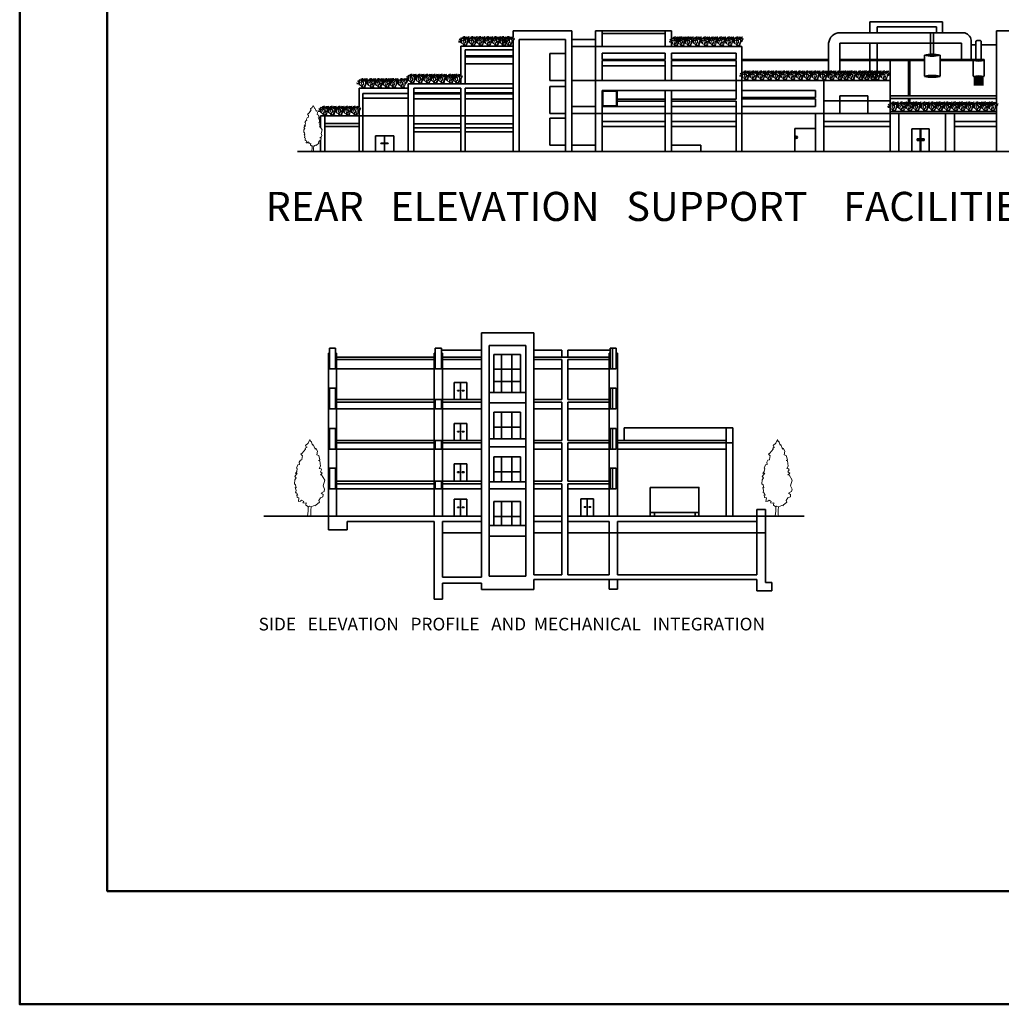
# Model space of a CAD drawing. Units: inches. Extents: x -1080 to 1950, y -1929 to 857.
# Tile 1 of 16: x -1080 to 294, y -1929 to -550. Entities that reach past the tile are written whole.
import ezdxf

# ---------------------------------------------------------------- set-up
doc = ezdxf.new("R2010")
doc.units = ezdxf.units.IN
doc.header["$MEASUREMENT"] = 0
for name, color, linetype, lineweight in [('A-ANNO-TEXT', 7, 'Continuous', 25), ('A-ANNO-TTLB', 7, 'Continuous', 50), ('A-ELEV', 7, 'Continuous', 35), ('L-PLNT', 82, 'Continuous', 13)]:
    doc.layers.add(name, color=color, linetype=linetype, lineweight=lineweight)
doc.styles.get("Standard").update_dxf_attribs({"font": 'arial.ttf'})

# ---------------------------------------------------------------- blocks, each defined once
blk = doc.blocks.new('*U6')
for p, q in [((-290.3982, 464.5406), (-265.6078, 577.8246)), ((-451.104, 219.456), (-601.0402, 303.8094)), ((-451.104, 219.456), (-587.4512, 234.2388)), ((-463.296, 280.416), (-552.577, 423.037)), ((-463.296, 280.416), (-512.064, 292.608)), ((-329.184, 316.992), (-499.872, 414.528)), ((-353.568, 316.992), (-487.68, 377.952)), ((-426.72, 414.528), (-475.488, 475.488)), ((-402.336, 207.264), (-463.296, 280.416)), ((-414.528, 182.88), (-463.296, 182.88)), ((-377.952, 463.296), (-451.104, 487.68)), ((-426.72, 316.992), (-451.104, 329.184)), ((-377.952, 146.304), (-451.104, 219.456)), ((-402.336, 12.192), (-451.104, 0)), ((-426.72, 414.528), (-390.144, 499.872)), ((-426.72, 316.992), (-426.72, 414.528)), ((-402.336, 207.264), (-426.72, 316.992)), ((-377.952, 146.304), (-402.336, 207.264)), ((-341.376, 12.192), (-402.336, 12.192)), ((-377.952, 463.296), (-329.184, 524.256)), ((-207.264, 304.8), (-377.952, 463.296)), ((-329.184, 121.92), (-377.952, 146.304)), ((-329.184, 316.992), (-353.568, 316.992)), ((-243.84, 24.384), (-341.376, 12.192)), ((-338.455, 424.7896), (-290.3982, 464.5406)), ((-329.184, 316.992), (-207.264, 451.104)), ((-268.224, 109.728), (-329.184, 316.992)), ((-292.608, 60.96), (-329.184, 121.92)), ((-243.84, 24.384), (-329.184, 0)), ((-316.7634, 502.285), (-327.6092, 559.9176)), ((-296.5958, 484.4034), (-316.7634, 502.285)), ((-286.512, 498.3226), (-307.4416, 538.0736)), ((-305.8922, 396.9512), (-302.7934, 478.4344)), ((-304.3428, 426.7708), (-268.7066, 458.5716)), ((-302.7934, 478.4344), (-270.256, 518.1854)), ((-219.456, 24.384), (-292.608, 60.96)), ((-268.7066, 458.5716), (-250.0884, 500.3038)), ((-207.264, 451.104), (-268.224, 548.64)), ((-268.224, 109.728), (-219.456, 195.072)), ((-219.456, 48.768), (-268.224, 109.728)), ((-243.84, 24.384), (-195.072, 24.384)), ((-240.792, 502.285), (-228.3968, 573.8368)), ((-182.88, 499.872), (-219.456, 512.064)), ((-219.456, 195.072), (-207.264, 304.8)), ((-219.456, 24.384), (-109.728, 73.152)), ((-219.456, 24.384), (-158.496, 73.152)), ((-219.456, 24.384), (-219.456, 48.768)), ((-219.456, 24.384), (-73.152, 24.384)), ((-207.264, 451.104), (-134.112, 487.68)), ((-195.072, 316.992), (-182.88, 377.952)), ((-170.688, 219.456), (-195.072, 316.992)), ((-195.072, 24.384), (-158.496, 12.192)), ((-182.88, 499.872), (-158.496, 536.448)), ((-121.92, 414.528), (-182.88, 499.872)), ((-182.88, 377.952), (-97.536, 426.72)), ((-146.304, 134.112), (-170.688, 219.456)), ((-158.496, 73.152), (-146.304, 134.112)), ((-158.496, 12.192), (-85.344, 0)), ((-129.1844, 450.6214), (-140.0302, 542.036)), ((-134.112, 487.68), (-97.536, 548.64)), ((-85.7758, 389.001), (-129.1844, 452.6026)), ((-73.152, 329.184), (-109.728, 499.872)), ((-109.728, 73.152), (-48.768, 243.84)), ((-97.536, 426.72), (-24.384, 524.256)), ((-85.7758, 472.4908), (-73.3552, 548.005)), ((-70.2564, 426.7708), (-85.7758, 472.4908)), ((-85.344, 134.112), (-73.152, 329.184)), ((-73.152, 402.336), (-60.96, 512.064)), ((-24.384, 268.224), (-73.152, 402.336)), ((-73.152, 24.384), (0, 0)), ((-48.768, 243.84), (24.384, 304.8)), ((-12.9032, 555.9552), (-2.0574, 522.1732)), ((-12.192, 274.32), (8.7884, 335.3562)), ((-5.1562, 486.3846), (2.5908, 542.036)), ((8.7884, 335.3562), (-5.1562, 486.3846)), ((-3.6068, 492.3536), (14.986, 518.1854)), ((-0.508, 508.254), (22.7584, 536.067)), ((1.0414, 526.1356), (35.1536, 559.9176)), ((2.5908, 542.036), (21.209, 555.9552)), ((8.7884, 335.3562), (33.6042, 412.8516)), ((24.384, 304.8), (36.576, 390.144)), ((24.384, 304.8), (73.152, 377.952)), ((33.6042, 412.8516), (92.5068, 464.5406)), ((36.576, 390.144), (73.152, 438.912)), ((48.768, 341.376), (60.96, 390.144)), ((60.96, 390.144), (85.344, 414.528))]:
    blk.add_line(p, q)
blk = doc.blocks.new('*U5')
blk.add_lwpolyline([(-2.754, 191.699), (-6.78, 182.851), (-13.682, 176.953), (-11.956, 173.266), (-9.656, 172.529), (-14.257, 170.317), (-13.682, 167.368), (-21.733, 157.783), (-25.184, 154.834), (-21.158, 150.41), (-21.733, 147.461), (-22.884, 140.825), (-26.334, 140.087), (-29.21, 134.926), (-28.635, 129.028), (-32.661, 128.291), (-36.111, 120.18), (-34.386, 118.706), (-35.536, 111.333), (-38.987, 106.171), (-34.386, 107.646), (-40.712, 98.798), (-37.261, 95.849), (-40.712, 90.688), (-41.287, 80.366), (-38.412, 78.154), (-36.686, 70.781), (-39.562, 71.518), (-37.261, 64.145), (-38.412, 57.509), (-36.111, 58.247), (-33.236, 52.348), (-35.536, 53.086), (-34.961, 46.45), (-30.36, 44.975), (-31.51, 36.128), (-26.334, 36.865), (-23.459, 39.814), (-18.283, 36.128), (-20.008, 33.178), (-14.832, 31.704), (-11.956, 33.178), (-12.531, 27.28), (-6.205, 22.856), (-3.905, 24.331), (0.121, 22.856), (8.173, 26.543), (11.624, 25.068), (12.199, 27.28), (21.4, 34.653), (19.675, 39.077), (23.701, 44.975), (30.027, 47.924), (30.602, 53.823), (25.426, 56.772), (32.903, 61.196), (34.053, 67.094), (30.602, 75.205), (34.628, 89.951), (26.576, 103.222), (23.701, 103.222), (28.302, 107.646), (23.701, 110.595), (26.576, 115.756), (25.426, 117.968), (20.825, 118.706), (24.276, 124.604), (22.551, 137.876), (19.1, 139.35), (22.551, 140.825), (19.675, 151.884), (14.499, 153.359), (16.224, 162.207), (12.199, 170.317), (10.473, 167.368), (5.872, 179.165), (4.147, 177.69), (0.696, 187.275), (-0.454, 185.8)], close=True)
for points in [[(-6.813, 23.669), (-6.813, 11.669), (-8.627, 0)], [(0.387, 23.669), (-0.576, 13.271), (-0.576, 3.686), (0, 0)]]:
    blk.add_lwpolyline(points)

msp = doc.modelspace()

# ---------------------------------------------------------------- linework, layer by layer
at = {"layer": 'A-ANNO-TTLB'}
for points in [[(-1080.1, 856.5), (1950.4, 856.5), (1950.4, -1929), (-1080.1, -1929)], [(-957.6, 743.5), (1813.4, 743.5), (1813.4, -1770.5), (-957.6, -1770.5)]]:
    msp.add_lwpolyline(points, close=True, dxfattribs=at)
at = {"layer": 'A-ELEV'}
for p, q in [((-307.2, -565.3), (-389.4, -565.3)), ((-389.4, -565.3), (-389.4, -573.8)), ((-307.2, -734.7), (-307.2, -565.3)), ((-274.1, -565.3), (-264.9, -565.3)), ((-274.1, -565.3), (-274.1, -577.5)), ((-274.1, -565.3), (-176.6, -565.3)), ((-264.9, -587.2), (-264.9, -565.3)), ((-176.6, -565.3), (-176.6, -577.5)), ((-167.5, -565.3), (-176.6, -565.3)), ((-167.5, -576.3), (-167.5, -565.3)), ((109.9, -552.8), (211.8, -552.8)), ((109.9, -567.9), (109.9, -552.8)), ((120, -567.9), (120, -559.8)), ((120, -559.8), (203, -559.8)), ((203, -559.8), (203, -567.9)), ((211.8, -552.8), (211.8, -567.9)), ((287.1, -565.3), (287.1, -606)), ((287.1, -565.3), (345.7, -565.3)), ((-389.4, -574.1), (-389.4, -574.7)), ((-389.4, -578.7), (-389.4, -578.9)), ((-380.8, -734.7), (-380.8, -577.5)), ((-380.8, -577.5), (-315.9, -577.5)), ((-315.9, -577.5), (-315.9, -734.7)), ((-307.2, -577.5), (-274.1, -577.5)), ((-274.1, -577.5), (-274.1, -587.2)), ((-264.9, -569.2), (-176.6, -569.2)), ((-176.6, -577.5), (-176.6, -587.2)), ((68, -568.1), (114.5, -568.1)), ((109.9, -567.9), (109.9, -568.1)), ((114.5, -568.1), (240.5, -568.1)), ((120, -567.9), (120, -567.9)), ((120, -567.9), (120, -568.1)), ((194.9, -568.1), (194.9, -599.6)), ((198.9, -568.1), (198.9, -599.6)), ((203, -567.9), (203, -568.1)), ((211.8, -567.9), (211.8, -568.1)), ((251.9, -578.8), (251.9, -605.7)), ((-462.5, -587), (-389.4, -587)), ((-462.5, -628.8), (-462.5, -587)), ((-389.4, -592), (-456.5, -592)), ((-456.5, -639.5), (-456.5, -592)), ((-456.5, -592), (-389.4, -592)), ((-455.2, -592), (-389.4, -592)), ((-389.4, -579.9), (-389.4, -587)), ((-389.4, -587), (-389.4, -592)), ((-389.4, -592), (-389.4, -734.7)), ((-307.2, -587.2), (-274.1, -587.2)), ((-274.1, -587.2), (-274.1, -734.7)), ((-274.1, -587.2), (-167.5, -587.2)), ((-167.5, -581.8), (-167.5, -587.2)), ((-167.5, -587.2), (-77.3, -587.2)), ((-69.5, -587.2), (-77.3, -587.2)), ((-69.5, -623.6), (-69.5, -587.2)), ((52.2, -623.6), (52.2, -582.7)), ((68.1, -582.7), (114.5, -582.7)), ((68.1, -623.9), (68.1, -582.7)), ((109.9, -582.7), (109.9, -623.7)), ((109.9, -582.7), (109.9, -585.8)), ((114.5, -582.7), (238.3, -582.7)), ((120, -582.7), (120, -623.5)), ((120, -582.7), (120, -585.8)), ((238.3, -582.7), (238.3, -605.7)), ((251.9, -585), (258.5, -585)), ((258.5, -588.2), (258.5, -579.9)), ((258.5, -605.7), (258.5, -588.2)), ((265.9, -579.9), (265.9, -588.2)), ((265.9, -585), (287.1, -585)), ((265.9, -588.2), (265.9, -605.7)), ((-456.5, -600.7), (-389.4, -600.7)), ((-456.5, -601.9), (-389.4, -601.9)), ((-315.9, -597.3), (-338.1, -597.3)), ((-338.1, -597.3), (-338.1, -635.1)), ((-264.9, -596.9), (-176.6, -596.9)), ((-264.9, -605.7), (-264.9, -596.9)), ((-264.9, -605.7), (-176.6, -605.7)), ((-176.6, -596.9), (-176.6, -605.7)), ((-167.5, -596.9), (-77.3, -596.9)), ((-167.5, -596.9), (-167.5, -605.7)), ((-167.5, -605.7), (-77.3, -605.7)), ((-77.3, -596.9), (-77.3, -605.7)), ((-69.5, -605.7), (52.2, -605.7)), ((68.1, -605.7), (166.1, -605.7)), ((138.3, -635.1), (138.3, -605.7)), ((166.1, -605.7), (166.1, -656.7)), ((166.1, -605.7), (186.3, -605.7)), ((194.9, -599.6), (186.3, -599.6)), ((186.3, -599.6), (186.3, -629.2)), ((194.9, -599.6), (208.3, -599.6)), ((208.3, -629.2), (208.3, -599.6)), ((208.3, -605.7), (264.9, -605.7)), ((254.5, -605.7), (254.5, -629.2)), ((269.9, -605.7), (264.9, -605.7)), ((269.9, -605.7), (269.9, -607.2)), ((287.1, -665.7), (287.1, -606)), ((-456.5, -611.5), (-389.4, -611.5)), ((-264.9, -635.1), (-264.9, -607.2)), ((-264.9, -607.2), (-176.6, -607.2)), ((-264.9, -614.5), (-176.6, -614.5)), ((-176.6, -607.2), (-176.6, -635.1)), ((-167.5, -607.2), (-77.3, -607.2)), ((-167.5, -607.2), (-167.5, -635.1)), ((-167.5, -614.5), (-77.3, -614.5)), ((-77.3, -607.2), (-77.3, -661.3)), ((-69.5, -607.2), (52.2, -607.2)), ((68.1, -607.2), (164.1, -607.2)), ((164.1, -607.2), (164.1, -656.7)), ((164.1, -607.2), (186.3, -607.2)), ((208.3, -607.2), (254.5, -607.2)), ((254.5, -607.2), (269.9, -607.2)), ((269.9, -629.2), (269.9, -607.2)), ((-462.5, -639.5), (-462.5, -632.1)), ((-69.5, -628.1), (-69.5, -627.8)), ((-69.5, -659), (-69.5, -629.3)), ((52.2, -630.9), (52.2, -626.5)), ((68.1, -629.3), (68.1, -628.1)), ((68.1, -635.1), (68.1, -633.8)), ((109.9, -626.5), (109.9, -631.3)), ((120, -624.3), (120, -630.1)), ((120, -634.3), (120, -635.1)), ((186.3, -629.2), (208.3, -629.2)), ((256.6, -628.9), (256.6, -642.2)), ((258.1, -628.9), (258.1, -642.2)), ((259.2, -628.9), (259.2, -642.2)), ((260.7, -628.9), (260.7, -642.2)), ((262, -628.9), (262, -642.2)), ((263.4, -628.9), (263.4, -642.2)), ((263.4, -628.9), (263.4, -642.2)), ((264.7, -628.9), (264.7, -642.2)), ((265.7, -628.9), (265.7, -642.2)), ((266.8, -628.9), (266.8, -642.2)), ((268, -628.9), (268, -642.2)), ((268, -628.9), (268, -642.2)), ((-604.9, -657.6), (-604.9, -645.6)), ((-604.9, -645.6), (-536.5, -645.6)), ((-536.5, -645.6), (-536.5, -639.5)), ((-536.5, -639.5), (-528.2, -639.5)), ((-536.5, -653.1), (-536.5, -645.6)), ((-528.2, -639.5), (-462.5, -639.5)), ((-528.2, -639.5), (-462.5, -639.5)), ((-528.2, -734.7), (-528.2, -645.6)), ((-528.2, -645.6), (-462.5, -645.6)), ((-528.2, -645.6), (-462.5, -645.6)), ((-462.5, -639.5), (-389.4, -639.5)), ((-462.5, -734.7), (-462.5, -645.6)), ((-456.5, -645.6), (-456.5, -734.7)), ((-456.5, -645.6), (-389.4, -645.6)), ((-338.1, -635.1), (-315.9, -635.1)), ((-315.9, -643.6), (-338.1, -643.6)), ((-338.1, -643.6), (-338.1, -681.3)), ((-307.2, -635.1), (-77.3, -635.1)), ((-77.3, -635.1), (113, -635.1)), ((45.4, -734.7), (45.4, -635.1)), ((52.2, -635.1), (52.2, -634.6)), ((109.9, -634.6), (109.9, -635.1)), ((113, -635.1), (138.3, -635.1)), ((138.3, -635.1), (138.3, -667.8)), ((-604.9, -657.6), (-604.9, -672.3)), ((-600, -734.7), (-600, -653.1)), ((-536.5, -653.1), (-600, -653.1)), ((-600, -659.7), (-536.5, -659.7)), ((-536.5, -653.1), (-536.5, -734.7)), ((-528.2, -652.3), (-462.5, -652.3)), ((-528.2, -653.7), (-462.5, -653.7)), ((-528.2, -660.9), (-462.5, -660.9)), ((-456.5, -652.3), (-389.4, -652.3)), ((-456.5, -653.7), (-389.4, -653.7)), ((-456.5, -660.9), (-389.4, -660.9)), ((-264.9, -734), (-264.9, -649.2)), ((-264.9, -649.2), (-77.3, -649.2)), ((-244, -671.6), (-244, -649.2)), ((-244, -661.3), (-176.6, -661.3)), ((-176.6, -649.2), (-176.6, -734.7)), ((-167.5, -649.2), (-167.5, -661.3)), ((-167.5, -661.3), (-77.3, -661.3)), ((-167.5, -661.3), (-167.5, -734.7)), ((-69.5, -649.2), (34, -649.2)), ((-69.5, -659), (34, -659)), ((-69.5, -660.9), (-69.5, -659)), ((-69.5, -734.7), (-69.5, -660.9)), ((-69.5, -660.9), (34, -660.9)), ((34, -649.2), (34, -659)), ((34, -660.9), (34, -671.6)), ((68, -681.3), (68, -656.4)), ((68, -656.4), (107, -656.4)), ((107, -656.4), (107, -681.3)), ((138.3, -656.7), (287.1, -656.7)), ((138.3, -660.1), (287.1, -660.1)), ((164.1, -660.1), (164.1, -666.5)), ((166.1, -660.1), (166.1, -666.2)), ((-307.2, -671.6), (-274.1, -671.6)), ((-264.9, -671.6), (-176.6, -671.6)), ((-176.6, -663.9), (-244, -663.9)), ((-167.5, -663.9), (-77.3, -663.9)), ((-167.5, -671.6), (-77.3, -671.6)), ((-77.3, -663.9), (-77.3, -734.7)), ((34, -671.6), (-69.5, -671.6)), ((45.4, -663.4), (138.3, -663.4)), ((138.3, -669.1), (138.3, -670.5)), ((138.3, -674), (138.3, -734.7)), ((164.1, -667.2), (164.1, -667.8)), ((287.1, -681.3), (287.1, -670.8)), ((-659, -684.4), (-653.2, -684.4)), ((-659, -700.7), (-659, -684.4)), ((-653.2, -684.4), (-653.2, -734.7)), ((-653.2, -684.4), (-604.9, -684.4)), ((-604.9, -677.4), (-604.9, -684.4)), ((-604.9, -684.4), (-604.9, -734.7)), ((-604.9, -684.4), (-600, -684.4)), ((-600, -684.5), (-528.2, -684.5)), ((-528.2, -684.5), (-462.5, -684.5)), ((-462.5, -684.5), (-456.5, -684.5)), ((-456.5, -684.5), (-389.4, -684.5)), ((-338.1, -681.3), (-315.9, -681.3)), ((-315.9, -687.9), (-338.1, -687.9)), ((-338.1, -687.9), (-338.1, -725.6)), ((-307.2, -681.3), (-264.9, -681.3)), ((-264.9, -681.3), (-77.3, -681.3)), ((-77.3, -681.3), (93.5, -681.3)), ((34, -681.3), (34, -734.7)), ((93.5, -681.3), (138.3, -681.3)), ((138.3, -678.4), (287.1, -678.4)), ((138.3, -681.3), (228.4, -681.3)), ((150.7, -681.3), (150.7, -734.7)), ((164.1, -676.9), (164.1, -678.4)), ((166.1, -677.5), (166.1, -678.4)), ((215.6, -681.3), (215.6, -734.7)), ((228.4, -681.3), (228.4, -734.7)), ((228.4, -681.3), (287.1, -681.3)), ((287.1, -681.3), (287.1, -734.7)), ((-653.2, -695.5), (-604.9, -695.5)), ((-653.2, -699.7), (-604.9, -699.7)), ((-528.2, -695.7), (-462.5, -695.7)), ((-528.2, -701.4), (-462.5, -701.4)), ((-456.5, -695.7), (-389.4, -695.7)), ((-456.5, -701.4), (-389.4, -701.4)), ((-264.7, -692.6), (-176.6, -692.6)), ((-264.7, -699.5), (-176.6, -699.5)), ((-167.5, -692.6), (-77.3, -692.6)), ((-167.5, -699.5), (-77.3, -699.5)), ((34, -702.4), (4.7, -702.4)), ((4.7, -702.4), (4.7, -734.7)), ((45.4, -692.6), (138.3, -692.6)), ((45.4, -699.5), (138.3, -699.5)), ((168.5, -734.7), (168.5, -702.6)), ((168.5, -702.6), (192.9, -702.6)), ((180.3, -702.6), (180.3, -734.7)), ((181.2, -702.6), (181.2, -734.7)), ((192.9, -702.6), (192.9, -734.7)), ((228.4, -692.6), (287.1, -692.6)), ((228.4, -699.5), (287.1, -699.5)), ((-659, -716), (-659, -714.9)), ((-582.1, -734.7), (-582.1, -712.4)), ((-582.1, -712.4), (-556.3, -712.4)), ((-569.3, -712.4), (-569.3, -734.7)), ((-556.3, -712.4), (-556.3, -734.7)), ((-528.2, -707), (-462.5, -707)), ((-456.5, -707), (-389.4, -707)), ((6.9, -714.5), (7.7, -714.5)), ((176, -716.8), (176, -719.3)), ((179.7, -716.8), (176, -716.8)), ((179.7, -719.3), (179.7, -716.8)), ((182.1, -716.8), (182.1, -719.3)), ((185.9, -716.8), (182.1, -716.8)), ((185.9, -719.3), (185.9, -716.8)), ((-659, -718.2), (-659, -734.7)), ((-659, -734.7), (-659, -718.7)), ((-574.4, -723.5), (-574.4, -722.7)), ((-574.4, -722.7), (-573.3, -722.7)), ((-570.8, -723.5), (-574.4, -723.5)), ((-573.3, -722.7), (-570.8, -722.7)), ((-570.8, -722.7), (-570.8, -723.5)), ((-568.1, -723.5), (-568.1, -722.7)), ((-568.1, -722.7), (-566.9, -722.7)), ((-564.4, -723.5), (-568.1, -723.5)), ((-566.9, -722.7), (-564.4, -722.7)), ((-564.4, -722.7), (-564.4, -723.5)), ((-338.1, -725.6), (-315.9, -725.6)), ((-307.2, -725.6), (-274.1, -725.6)), ((-167.5, -725.6), (-126.7, -725.6)), ((-126.7, -725.6), (-126.7, -734.7)), ((176, -719.3), (179.7, -719.3)), ((182.1, -719.3), (185.9, -719.3)), ((-691.1, -734.7), (-262.7, -734.7)), ((-262.7, -734.7), (342.8, -734.7)), ((-433.5, -1258.6), (-433.5, -988.5)), ((-433.5, -988.5), (-360.3, -988.5)), ((-360.3, -988.5), (-360.3, -1327.4)), ((-422.8, -1329.4), (-422.8, -1006.4)), ((-422.8, -1006.4), (-371.6, -1006.4)), ((-371.6, -1006.4), (-371.6, -1329.4)), ((-647.8, -1245.3), (-647.8, -1017.1)), ((-647.8, -1017.1), (-646.5, -1017.1)), ((-646.5, -1017.1), (-646.5, -1009.9)), ((-646.5, -1009.9), (-638, -1009.9)), ((-646.5, -1017.1), (-646.5, -1038.8)), ((-638, -1009.9), (-638, -1017.1)), ((-638, -1038.8), (-638, -1017.1)), ((-638, -1017.1), (-636.5, -1017.1)), ((-636.5, -1017.1), (-636.5, -1245.3)), ((-499.7, -1245.3), (-499.7, -1017.1)), ((-499.7, -1017.1), (-498.4, -1017.1)), ((-498.4, -1017.1), (-498.4, -1009.9)), ((-498.4, -1009.9), (-489.9, -1009.9)), ((-498.4, -1017.1), (-498.4, -1038.8)), ((-489.9, -1009.9), (-489.9, -1017.1)), ((-489.9, -1012.9), (-433.5, -1012.9)), ((-489.9, -1017.1), (-488.3, -1017.1)), ((-489.9, -1038.8), (-489.9, -1017.1)), ((-488.3, -1017.1), (-488.3, -1245.3)), ((-416.3, -1072), (-416.3, -1018.6)), ((-416.3, -1018.6), (-379.2, -1018.6)), ((-405.8, -1018.6), (-405.8, -1072)), ((-391.4, -1018.6), (-391.4, -1072)), ((-379.2, -1018.6), (-379.2, -1072.2)), ((-360.3, -1012.9), (-321.1, -1012.9)), ((-321.1, -1012.9), (-321.1, -1022.5)), ((-312.8, -1012.9), (-312.8, -1022.5)), ((-312.8, -1012.9), (-253.6, -1012.9)), ((-254.9, -1245.3), (-254.9, -1017.1)), ((-254.9, -1017.1), (-253.6, -1017.1)), ((-253.6, -1017.1), (-253.6, -1009.9)), ((-253.6, -1009.9), (-245.1, -1009.9)), ((-253.6, -1017.1), (-253.6, -1038.8)), ((-250.1, -1009.9), (-250.1, -1038.8)), ((-245.1, -1009.9), (-245.1, -1017.1)), ((-245.1, -1017.1), (-243.5, -1017.1)), ((-245.1, -1038.8), (-245.1, -1017.1)), ((-243.5, -1017.1), (-243.5, -1245.3)), ((-636.5, -1022.5), (-498.4, -1022.5)), ((-636.5, -1025.8), (-498.4, -1025.8)), ((-489.9, -1022.5), (-433.5, -1022.5)), ((-489.9, -1025.8), (-433.5, -1025.8)), ((-360.3, -1022.5), (-321.1, -1022.5)), ((-360.3, -1025.8), (-321.1, -1025.8)), ((-321.1, -1022.5), (-312.8, -1022.5)), ((-321.1, -1025.8), (-321.1, -1082)), ((-312.8, -1022.5), (-254.9, -1022.5)), ((-312.8, -1025.8), (-254.9, -1025.8)), ((-312.8, -1025.8), (-312.8, -1082)), ((-646.5, -1038.8), (-638, -1038.8)), ((-638, -1038.8), (-433.5, -1038.8)), ((-498.4, -1038.8), (-489.9, -1038.8)), ((-416.3, -1039.3), (-379.2, -1039.3)), ((-360.3, -1038.8), (-321.1, -1038.8)), ((-312.8, -1038.8), (-254.9, -1038.8)), ((-253.6, -1038.8), (-245.1, -1038.8)), ((-471.8, -1082), (-471.8, -1058)), ((-471.8, -1058), (-454.2, -1058)), ((-462.9, -1082), (-462.9, -1058)), ((-454.2, -1058), (-454.2, -1082)), ((-416.3, -1056.7), (-379.2, -1056.7)), ((-646.5, -1073.3), (-646.5, -1066.1)), ((-646.5, -1066.1), (-638, -1066.1)), ((-646.5, -1073.3), (-646.5, -1095)), ((-638, -1066.1), (-638, -1073.3)), ((-638, -1095), (-638, -1073.3)), ((-467.4, -1069.1), (-467.4, -1069.8)), ((-464.8, -1069.1), (-467.4, -1069.1)), ((-467.4, -1069.8), (-464.8, -1069.8)), ((-464.8, -1069.8), (-464.8, -1069.1)), ((-460.7, -1069.1), (-460.7, -1069.8)), ((-458.1, -1069.1), (-460.7, -1069.1)), ((-460.7, -1069.8), (-458.1, -1069.8)), ((-458.1, -1069.8), (-458.1, -1069.1)), ((-422.8, -1072), (-371.6, -1072)), ((-253.6, -1073.3), (-253.6, -1066.1)), ((-253.6, -1066.1), (-245.1, -1066.1)), ((-253.6, -1073.3), (-253.6, -1095)), ((-250.1, -1066.1), (-250.1, -1095)), ((-245.1, -1066.1), (-245.1, -1073.3)), ((-245.1, -1095), (-245.1, -1073.3)), ((-636.5, -1082), (-499.7, -1082)), ((-636.5, -1085.5), (-499.7, -1085.5)), ((-498.4, -1082), (-498.4, -1095)), ((-498.4, -1082), (-489.9, -1082)), ((-489.9, -1095), (-489.9, -1082)), ((-488.3, -1082), (-433.5, -1082)), ((-488.3, -1085.5), (-433.5, -1085.5)), ((-422.8, -1086.5), (-371.6, -1086.5)), ((-360.3, -1082), (-321.1, -1082)), ((-360.3, -1085.5), (-321.1, -1085.5)), ((-321.1, -1085.5), (-321.1, -1139.5)), ((-312.8, -1082), (-254.9, -1082)), ((-312.8, -1085.5), (-254.9, -1085.5)), ((-312.8, -1085.5), (-312.8, -1139.5)), ((-646.5, -1095), (-638, -1095)), ((-638, -1095), (-499.7, -1095)), ((-498.4, -1095), (-489.9, -1095)), ((-498.4, -1095), (-489.9, -1095)), ((-488.3, -1095), (-433.5, -1095)), ((-416.3, -1099.8), (-379.2, -1099.8)), ((-416.3, -1137.1), (-416.3, -1099.8)), ((-405.8, -1099.8), (-405.8, -1137.1)), ((-391.4, -1099.8), (-391.4, -1137.1)), ((-379.2, -1099.8), (-379.2, -1137.1)), ((-360.3, -1095), (-321.1, -1095)), ((-312.8, -1095), (-254.9, -1095)), ((-253.6, -1095), (-245.1, -1095)), ((-471.8, -1139.5), (-471.8, -1115.5)), ((-471.8, -1115.5), (-454.2, -1115.5)), ((-462.9, -1139.5), (-462.9, -1115.5)), ((-454.2, -1115.5), (-454.2, -1139.5)), ((-646.5, -1129.5), (-646.5, -1122.3)), ((-646.5, -1122.3), (-638, -1122.3)), ((-646.5, -1129.5), (-646.5, -1151.2)), ((-638, -1122.3), (-638, -1129.5)), ((-638, -1151.2), (-638, -1129.5)), ((-467.4, -1126.6), (-467.4, -1127.3)), ((-464.8, -1126.6), (-467.4, -1126.6)), ((-467.4, -1127.3), (-464.8, -1127.3)), ((-464.8, -1127.3), (-464.8, -1126.6)), ((-460.7, -1126.6), (-460.7, -1127.3)), ((-458.1, -1126.6), (-460.7, -1126.6)), ((-460.7, -1127.3), (-458.1, -1127.3)), ((-458.1, -1127.3), (-458.1, -1126.6)), ((-416.3, -1120.5), (-379.2, -1120.5)), ((-253.6, -1129.5), (-253.6, -1122.3)), ((-253.6, -1122.3), (-245.1, -1122.3)), ((-253.6, -1129.5), (-253.6, -1151.2)), ((-250.1, -1122.3), (-250.1, -1151.2)), ((-245.1, -1122.3), (-245.1, -1129.5)), ((-245.1, -1151.2), (-245.1, -1129.5)), ((-234.2, -1139.3), (-234.2, -1121.4)), ((-234.2, -1121.4), (-81.7, -1121.4)), ((-91.3, -1124.9), (-91.3, -1121.4)), ((-91.3, -1142.7), (-91.3, -1124.9)), ((-81.7, -1121.4), (-81.7, -1124.9)), ((-81.7, -1124.9), (-81.7, -1245.3)), ((-636.5, -1139.5), (-499.7, -1139.5)), ((-636.5, -1142.7), (-499.7, -1142.7)), ((-498.4, -1139.5), (-498.4, -1151.2)), ((-498.4, -1139.5), (-489.9, -1139.5)), ((-489.9, -1151.2), (-489.9, -1139.5)), ((-488.3, -1139.5), (-433.5, -1139.5)), ((-488.3, -1142.7), (-433.5, -1142.7)), ((-422.8, -1137.1), (-371.6, -1137.1)), ((-360.3, -1139.5), (-321.1, -1139.5)), ((-360.3, -1142.7), (-321.1, -1142.7)), ((-321.1, -1142.7), (-321.1, -1196.1)), ((-312.8, -1139.5), (-254.9, -1139.5)), ((-312.8, -1142.7), (-254.9, -1142.7)), ((-312.8, -1142.7), (-312.8, -1196.1)), ((-243.5, -1139.3), (-178.2, -1139.3)), ((-243.5, -1142.7), (-91.3, -1142.7)), ((-178.2, -1139.3), (-91.3, -1139.3)), ((-91.3, -1142.7), (-81.7, -1142.7)), ((-91.3, -1142.7), (-91.3, -1245.3)), ((-646.5, -1151.2), (-638, -1151.2)), ((-638, -1151.2), (-499.7, -1151.2)), ((-498.4, -1151.2), (-489.9, -1151.2)), ((-498.4, -1151.2), (-489.9, -1151.2)), ((-488.3, -1151.2), (-433.5, -1151.2)), ((-422.8, -1148.2), (-371.6, -1148.2)), ((-360.3, -1151.2), (-321.1, -1151.2)), ((-312.8, -1151.2), (-254.9, -1151.2)), ((-253.6, -1151.2), (-245.1, -1151.2)), ((-243.5, -1151.2), (-91.3, -1151.2)), ((-471.8, -1196.1), (-471.8, -1172.1)), ((-471.8, -1172.1), (-454.2, -1172.1)), ((-462.9, -1196.1), (-462.9, -1172.1)), ((-454.2, -1172.1), (-454.2, -1196.1)), ((-416.3, -1197.2), (-416.3, -1162.3)), ((-416.3, -1162.3), (-379.2, -1162.3)), ((-405.8, -1162.3), (-405.8, -1197.2)), ((-391.4, -1162.3), (-391.4, -1197.2)), ((-379.2, -1162.3), (-379.2, -1197.2)), ((-646.5, -1185), (-646.5, -1177.8)), ((-646.5, -1177.8), (-638, -1177.8)), ((-646.5, -1185), (-646.5, -1206.8)), ((-638, -1177.8), (-638, -1185)), ((-638, -1206.8), (-638, -1185)), ((-467.4, -1183.2), (-467.4, -1183.9)), ((-464.8, -1183.2), (-467.4, -1183.2)), ((-467.4, -1183.9), (-464.8, -1183.9)), ((-464.8, -1183.9), (-464.8, -1183.2)), ((-460.7, -1183.2), (-460.7, -1183.9)), ((-458.1, -1183.2), (-460.7, -1183.2)), ((-460.7, -1183.9), (-458.1, -1183.9)), ((-458.1, -1183.9), (-458.1, -1183.2)), ((-416.3, -1183), (-379.2, -1183)), ((-253.6, -1185), (-253.6, -1177.8)), ((-253.6, -1177.8), (-245.1, -1177.8)), ((-253.6, -1185), (-253.6, -1206.8)), ((-250.1, -1177.8), (-250.1, -1206.8)), ((-245.1, -1177.8), (-245.1, -1185)), ((-245.1, -1206.8), (-245.1, -1185)), ((-636.5, -1196.1), (-499.7, -1196.1)), ((-498.4, -1196.1), (-498.4, -1206.8)), ((-498.4, -1196.1), (-489.9, -1196.1)), ((-489.9, -1206.8), (-489.9, -1196.1)), ((-488.3, -1196.1), (-433.5, -1196.1)), ((-422.8, -1197.2), (-371.6, -1197.2)), ((-360.3, -1196.1), (-321.1, -1196.1)), ((-312.8, -1196.1), (-254.9, -1196.1)), ((-646.5, -1206.8), (-638, -1206.8)), ((-638, -1206.8), (-499.7, -1206.8)), ((-636.5, -1200), (-499.7, -1200)), ((-498.4, -1206.8), (-489.9, -1206.8)), ((-498.4, -1206.8), (-489.9, -1206.8)), ((-488.3, -1200), (-433.5, -1200)), ((-488.3, -1206.8), (-433.5, -1206.8)), ((-422.8, -1207), (-371.6, -1207)), ((-360.3, -1200), (-321.1, -1200)), ((-360.3, -1206.8), (-321.1, -1206.8)), ((-321.1, -1200), (-321.1, -1245.3)), ((-312.8, -1200), (-254.9, -1200)), ((-312.8, -1200), (-312.8, -1245.3)), ((-312.8, -1206.8), (-254.9, -1206.8)), ((-253.6, -1206.8), (-245.1, -1206.8)), ((-471.8, -1245.3), (-471.8, -1221.4)), ((-471.8, -1221.4), (-454.2, -1221.4)), ((-462.9, -1245.3), (-462.9, -1221.4)), ((-454.2, -1221.4), (-454.2, -1245.3)), ((-416.3, -1224.8), (-379.2, -1224.8)), ((-416.3, -1258.2), (-416.3, -1224.8)), ((-405.8, -1224.8), (-405.8, -1258.2)), ((-391.4, -1224.8), (-391.4, -1258.2)), ((-379.2, -1224.8), (-379.2, -1258.2)), ((-294.5, -1244.9), (-294.5, -1220.9)), ((-294.5, -1220.9), (-276.9, -1220.9)), ((-285.6, -1244.9), (-285.6, -1220.9)), ((-276.9, -1220.9), (-276.9, -1244.9)), ((-467.4, -1232.5), (-467.4, -1233.1)), ((-464.8, -1232.5), (-467.4, -1232.5)), ((-467.4, -1233.1), (-464.8, -1233.1)), ((-464.8, -1233.1), (-464.8, -1232.5)), ((-460.7, -1232.5), (-460.7, -1233.1)), ((-458.1, -1232.5), (-460.7, -1232.5)), ((-460.7, -1233.1), (-458.1, -1233.1)), ((-458.1, -1233.1), (-458.1, -1232.5)), ((-290.2, -1232), (-290.2, -1232.7)), ((-287.5, -1232), (-290.2, -1232)), ((-290.2, -1232.7), (-287.5, -1232.7)), ((-287.5, -1232.7), (-287.5, -1232)), ((-283.4, -1232), (-283.4, -1232.7)), ((-280.8, -1232), (-283.4, -1232)), ((-283.4, -1232.7), (-280.8, -1232.7)), ((-280.8, -1232.7), (-280.8, -1232)), ((-197.8, -1240.1), (-197.8, -1245.3)), ((-191.7, -1240.1), (-191.7, -1245.3)), ((-134.4, -1240.1), (-134.4, -1245.3)), ((-129.6, -1240.1), (-129.6, -1245.3)), ((-48.4, -1268.8), (-48.4, -1236)), ((-48.4, -1236), (-36.2, -1236)), ((-36.2, -1268.8), (-36.2, -1236)), ((-665.4, -1245.3), (-738.2, -1245.3)), ((-665.4, -1245.3), (-433.5, -1245.3)), ((-647.8, -1245.3), (-647.8, -1264.3)), ((-621.6, -1264.3), (-621.6, -1252.5)), ((-621.6, -1252.5), (-499.7, -1252.5)), ((-499.7, -1252.5), (-499.7, -1339.2)), ((-488.3, -1252.5), (-488.3, -1330.5)), ((-488.3, -1252.5), (-433.5, -1252.5)), ((-416.3, -1245.5), (-379.2, -1245.5)), ((-360.3, -1245.3), (-321.1, -1245.3)), ((-360.3, -1252.5), (-321.1, -1252.5)), ((-321.1, -1327.4), (-321.1, -1245.3)), ((-312.8, -1245.3), (-312.8, -1327.4)), ((-312.8, -1245.3), (-254.9, -1245.3)), ((-312.8, -1252.5), (-254.9, -1252.5)), ((-254.9, -1245.3), (-243.5, -1245.3)), ((-254.9, -1252.5), (-254.9, -1327.4)), ((-243.5, -1245.3), (-48.4, -1245.3)), ((-243.5, -1252.5), (-243.5, -1327.4)), ((-243.5, -1252.5), (-48.4, -1252.5)), ((-48.4, -1245.3), (18, -1245.3)), ((-647.8, -1264.3), (-621.6, -1264.3)), ((-433.5, -1258.6), (-433.5, -1330.5)), ((-422.8, -1258.2), (-371.6, -1258.2)), ((-488.3, -1268.8), (-433.5, -1268.8)), ((-422.8, -1273.2), (-371.6, -1273.2)), ((-360.1, -1268.8), (-321.1, -1268.8)), ((-312.8, -1268.8), (-305.2, -1268.8)), ((-305.2, -1268.8), (-254.9, -1268.8)), ((-254.9, -1268.8), (-243.5, -1268.8)), ((-243.5, -1268.8), (-36.2, -1268.8)), ((-48.4, -1268.8), (-48.4, -1327.4)), ((-36.2, -1268.8), (-36.2, -1334.2)), ((-488.3, -1330.5), (-433.5, -1330.5)), ((-371.6, -1329.4), (-422.8, -1329.4)), ((-360.3, -1327.4), (-321.1, -1327.4)), ((-312.8, -1334.2), (-360.3, -1334.2)), ((-360.3, -1334.2), (-360.3, -1347.9)), ((-321.1, -1327.4), (-338.7, -1327.4)), ((-254.9, -1327.4), (-312.8, -1327.4)), ((-243.5, -1334.2), (-312.8, -1334.2)), ((-254.9, -1334.2), (-254.9, -1347.7)), ((-48.4, -1327.4), (-243.5, -1327.4)), ((-48.4, -1334.2), (-243.5, -1334.2)), ((-243.5, -1347.7), (-243.5, -1334.2)), ((-48.4, -1334.2), (-48.4, -1349.9)), ((-36.2, -1338.1), (-36.2, -1334.2)), ((-499.7, -1361.6), (-499.7, -1339.2)), ((-488.3, -1339.2), (-433.5, -1339.2)), ((-488.3, -1339.2), (-488.3, -1361.6)), ((-433.5, -1339.2), (-433.5, -1347.9)), ((-433.5, -1347.9), (-422.8, -1347.9)), ((-422.8, -1347.9), (-360.3, -1347.9)), ((-254.9, -1347.7), (-243.5, -1347.7)), ((-48.4, -1349.9), (-27.3, -1349.9)), ((-27.3, -1338.1), (-36.2, -1338.1)), ((-27.3, -1349.9), (-27.3, -1338.1)), ((-488.3, -1361.6), (-499.7, -1361.6))]:
    msp.add_line(p, q, dxfattribs=at)
for points in [[(-264, -650.2), (-244.9, -650.2), (-244.9, -670.3), (-264, -670.3)], [(-197.8, -1205), (-129.4, -1205), (-129.4, -1240.1), (-197.8, -1240.1)]]:
    msp.add_lwpolyline(points, close=True, dxfattribs=at)
msp.add_circle((7, -714.5), 1.56, dxfattribs=at)
for centre, radius, start, end in [((68, -584), 15.8, 89.819, 175.4441), ((239.4, -580.7), 12.7, 8.8927, 84.8874), ((262.2, -585.9), 7.05, 58.2311, 121.7689), ((197.3, -642), 43.8, 75.4212, 104.5788), ((197.3, -550), 50.8, 257.4696, 282.5304), ((262.2, -641.8), 35.5, 77.4126, 102.5874), ((262.2, -557.2), 50.6, 261.2192, 278.7808), ((197.3, -675.9), 48, 76.7279, 103.2721), ((197.3, -585.7), 44.9, 255.771, 284.229), ((262.2, -687.4), 58.7, 82.4367, 97.5633), ((262.2, -599.9), 30.3, 255.2111, 284.7889)]:
    msp.add_arc(centre, radius, start, end, dxfattribs=at)

# ---------------------------------------------------------------- block references
at = {"layer": 'L-PLNT'}
for name, p, xscale, yscale, zscale in [('*U6', (-451.6, -586.9), 0.0240303115076123, 0.0240303115076123, 0.0240303115076123), ('*U6', (-440.2, -586.9), 0.0240303115076123, 0.0240303115076123, 0.0240303115076123), ('*U6', (-429.4, -586.9), 0.0240303115076123, 0.0240303115076123, 0.0240303115076123), ('*U6', (-418.5, -586.9), 0.0240303115076123, 0.0240303115076123, 0.0240303115076123), ('*U6', (-407.8, -586.9), 0.0240303115076123, 0.0240303115076123, 0.0240303115076123), ('*U6', (-397.2, -586.9), 0.0240303115076123, 0.0240303115076123, 0.0240303115076123), ('*U6', (-389.6, -586.9), 0.0240303115076123, 0.0240303115076123, 0.0240303115076123), ('*U6', (-156.6, -587.1), 0.0240303115076123, 0.0240303115076123, 0.0240303115076123), ('*U6', (-147.9, -587.1), 0.0240303115076123, 0.0240303115076123, 0.0240303115076123), ('*U6', (-137.9, -587.1), 0.0240303115076123, 0.0240303115076123, 0.0240303115076123), ('*U6', (-126.5, -587.1), 0.0240303115076123, 0.0240303115076123, 0.0240303115076123), ('*U6', (-114.7, -587.1), 0.0240303115076123, 0.0240303115076123, 0.0240303115076123), ('*U6', (-103.7, -587.1), 0.0240303115076123, 0.0240303115076123, 0.0240303115076123), ('*U6', (-92.4, -587.1), 0.0240303115076123, 0.0240303115076123, 0.0240303115076123), ('*U6', (-81.1, -587.1), 0.0240303115076123, 0.0240303115076123, 0.0240303115076123), ('*U6', (-69.4, -587.1), 0.0240303115076123, 0.0240303115076123, 0.0240303115076123), ('*U6', (-594.1, -645.5), 0.0240303115076123, 0.0240303115076123, 0.0240303115076123), ('*U6', (-582.3, -645.5), 0.0240303115076123, 0.0240303115076123, 0.0240303115076123), ('*U6', (-571.5, -645.5), 0.0240303115076123, 0.0240303115076123, 0.0240303115076123), ('*U6', (-560.9, -645.5), 0.0240303115076123, 0.0240303115076123, 0.0240303115076123), ('*U6', (-551.2, -645.5), 0.0240303115076123, 0.0240303115076123, 0.0240303115076123), ('*U6', (-539.1, -645.5), 0.0240303115076123, 0.0240303115076123, 0.0240303115076123), ('*U6', (-525.6, -639.5), 0.0240303115076123, 0.0240303115076123, 0.0240303115076123), ('*U6', (-514.5, -639.5), 0.0240303115076123, 0.0240303115076123, 0.0240303115076123), ('*U6', (-503.6, -639.5), 0.0240303115076123, 0.0240303115076123, 0.0240303115076123), ('*U6', (-493.3, -639.5), 0.0240303115076123, 0.0240303115076123, 0.0240303115076123), ('*U6', (-483.3, -639.5), 0.0240303115076123, 0.0240303115076123, 0.0240303115076123), ('*U6', (-471.6, -639.5), 0.0240303115076123, 0.0240303115076123, 0.0240303115076123), ('*U6', (-462.5, -639.5), 0.0240303115076123, 0.0240303115076123, 0.0240303115076123), ('*U6', (-58.2, -634.8), 0.0240303115076123, 0.0240303115076123, 0.0240303115076123), ('*U6', (-47.2, -634.8), 0.0240303115076123, 0.0240303115076123, 0.0240303115076123), ('*U6', (-36.1, -634.8), 0.0240303115076123, 0.0240303115076123, 0.0240303115076123), ('*U6', (-25.4, -634.8), 0.0240303115076123, 0.0240303115076123, 0.0240303115076123), ('*U6', (-14.6, -634.8), 0.0240303115076123, 0.0240303115076123, 0.0240303115076123), ('*U6', (-3.9, -634.8), 0.0240303115076123, 0.0240303115076123, 0.0240303115076123), ('*U6', (7, -634.8), 0.0240303115076123, 0.0240303115076123, 0.0240303115076123), ('*U6', (17.8, -634.8), 0.0240303115076123, 0.0240303115076123, 0.0240303115076123), ('*U6', (28.7, -634.8), 0.0240303115076123, 0.0240303115076123, 0.0240303115076123), ('*U6', (39.6, -634.8), 0.0240303115076123, 0.0240303115076123, 0.0240303115076123), ('*U6', (51, -634.8), 0.0240303115076123, 0.0240303115076123, 0.0240303115076123), ('*U6', (61.8, -634.8), 0.0240303115076123, 0.0240303115076123, 0.0240303115076123), ('*U6', (72.8, -634.8), 0.0240303115076123, 0.0240303115076123, 0.0240303115076123), ('*U6', (81.6, -634.8), 0.0240303115076123, 0.0240303115076123, 0.0240303115076123), ('*U6', (90.6, -634.8), 0.0240303115076123, 0.0240303115076123, 0.0240303115076123), ('*U6', (102.1, -634.8), 0.0240303115076123, 0.0240303115076123, 0.0240303115076123), ('*U6', (110.5, -634.8), 0.0240303115076123, 0.0240303115076123, 0.0240303115076123), ('*U6', (119.1, -634.8), 0.0240303115076123, 0.0240303115076123, 0.0240303115076123), ('*U6', (125.2, -634.8), 0.0240303115076123, 0.0240303115076123, 0.0240303115076123), ('*U6', (135.8, -634.8), 0.0240303115076123, 0.0240303115076123, 0.0240303115076123), ('*U5', (-668.6, -734.6), 0.3373382957572102, 0.3373382957572102, 0.3373382957572102), ('*U6', (-648.1, -684.3), 0.0240303115076123, 0.0240303115076123, 0.0240303115076123), ('*U6', (-637.4, -684.3), 0.0240303115076123, 0.0240303115076123, 0.0240303115076123), ('*U6', (-626.5, -684.3), 0.0240303115076123, 0.0240303115076123, 0.0240303115076123), ('*U6', (-615.7, -684.3), 0.0240303115076123, 0.0240303115076123, 0.0240303115076123), ('*U6', (-604.9, -684.3), 0.0240303115076123, 0.0240303115076123, 0.0240303115076123), ('*U6', (149, -678.4), 0.0240303115076123, 0.0240303115076123, 0.0240303115076123), ('*U6', (160.8, -678.4), 0.0240303115076123, 0.0240303115076123, 0.0240303115076123), ('*U6', (171.1, -678.4), 0.0240303115076123, 0.0240303115076123, 0.0240303115076123), ('*U6', (181.1, -678.4), 0.0240303115076123, 0.0240303115076123, 0.0240303115076123), ('*U6', (192.6, -678.4), 0.0240303115076123, 0.0240303115076123, 0.0240303115076123), ('*U6', (203.7, -678.4), 0.0240303115076123, 0.0240303115076123, 0.0240303115076123), ('*U6', (213.9, -678.4), 0.0240303115076123, 0.0240303115076123, 0.0240303115076123), ('*U6', (224.5, -678.4), 0.0240303115076123, 0.0240303115076123, 0.0240303115076123), ('*U6', (235.1, -678.4), 0.0240303115076123, 0.0240303115076123, 0.0240303115076123), ('*U6', (245, -678.4), 0.0240303115076123, 0.0240303115076123, 0.0240303115076123), ('*U6', (255.3, -678.4), 0.0240303115076123, 0.0240303115076123, 0.0240303115076123), ('*U6', (266.7, -678.4), 0.0240303115076123, 0.0240303115076123, 0.0240303115076123), ('*U6', (277.1, -678.4), 0.0240303115076123, 0.0240303115076123, 0.0240303115076123), ('*U6', (287.1, -678.4), 0.0240303115076123, 0.0240303115076123, 0.0240303115076123), ('*U5', (-672.4, -1244.9), 0.5580597638333467, 0.5580597638333467, 0.5580597638333467), ('*U5', (-18, -1244.9), 0.5580597638333467, 0.5580597638333467, 0.5580597638333467)]:
    msp.add_blockref(name, p, dxfattribs=dict(at, xscale=xscale, yscale=yscale, zscale=zscale))

# ---------------------------------------------------------------- texts
at = {"layer": 'A-ANNO-TEXT'}
for s, height, p in [('REAR   ELEVATION   SUPPORT    FACILITIES', 40.793, (-735.9, -831.8)), ('SIDE   ELEVATION   PROFILE   AND  MECHANICAL   INTEGRATION', 17.769, (-745.7, -1405.3))]:
    msp.add_text(s, height=height, dxfattribs=at).set_placement(p)

doc.saveas('drawing.dxf')
